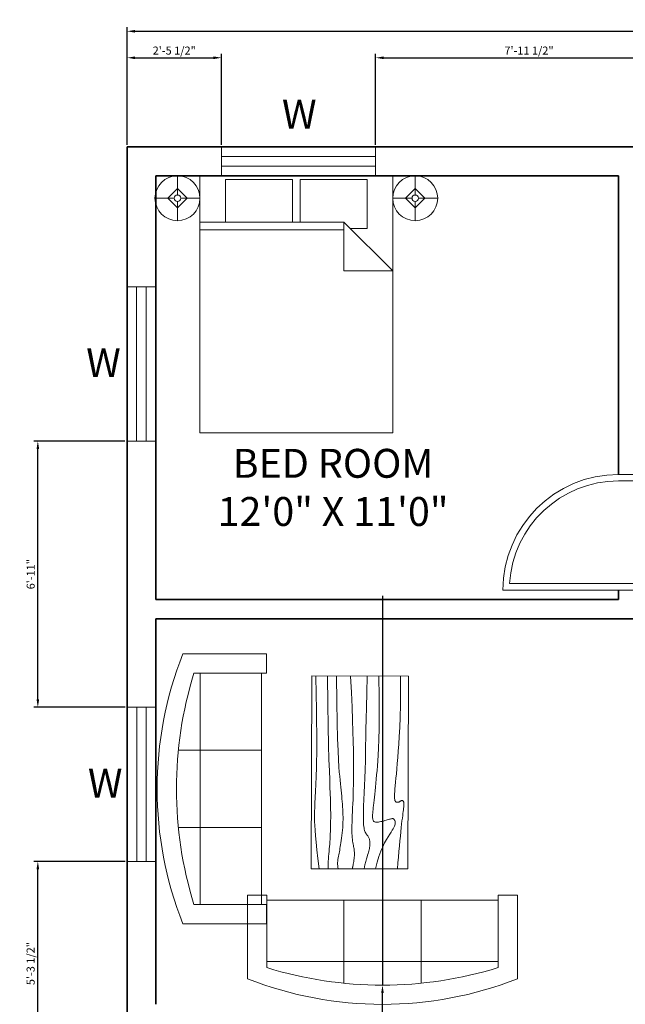
# Model space of a CAD drawing. Units: inches. Extents: x 1025 to 3479, y 1594 to 2212.
# Tile 2 of 9: x 1766 to 1954, y 1843 to 2150. Entities that reach past the tile are written whole.
import ezdxf

# ---------------------------------------------------------------- set-up
doc = ezdxf.new("R2010")
doc.units = ezdxf.units.IN
for name, color, linetype, lineweight in [('A-ANNO-DIMS', 1, 'Continuous', 18), ('A-ANNO-TEXT', 7, 'Continuous', 18), ('A-AREA-IDEN', 4, 'Continuous', 18), ('A-DOOR', 4, 'Continuous', 18), ('A-FURN', 8, 'Continuous', 13), ('A-GLAZ', 3, 'Continuous', 18), ('A-WALL', 7, 'Continuous', 35)]:
    doc.layers.add(name, color=color, linetype=linetype, lineweight=lineweight)
doc.styles.get("Standard").update_dxf_attribs({"font": 'arial.ttf'})
doc.dimstyles.new('ISO-25', dxfattribs={"dimtxt": 2.5, "dimasz": 2.5, "dimexe": 1.25, "dimexo": 0.625, "dimtad": 1, "dimdec": 0, "dimlunit": 3, "dimtxsty": 'Standard', "dimcen": 2.5, "dimadec": 0, "dimazin": 0, "dimtfac": 1, "dimtdec": 0, "dimtmove": 0, "dimatfit": 3, "dimfxl": 1, "dimarcsym": 0})

# ---------------------------------------------------------------- blocks, each defined once
blk = doc.blocks.new('*D1')
at = {"layer": 'A-ANNO-DIMS', "color": 0, "lineweight": -2, "transparency": 16777216}
for p, q in [((1799.1, 2111.11), (1799.1, 2147.74)), ((1801.6, 2146.49), (2156.6, 2146.49)), ((2159.1, 2111.11), (2159.1, 2147.74))]:
    blk.add_line(p, q, dxfattribs=at)
at = {"layer": 'A-ANNO-DIMS', "color": 0, "transparency": 16777216}
for points in [[(1801.6, 2146.9), (1801.6, 2146.07), (1799.1, 2146.49)], [(2156.6, 2146.9), (2156.6, 2146.07), (2159.1, 2146.49)]]:
    blk.add_solid(points, dxfattribs=at)
at = {"layer": 'Defpoints', "color": 0, "transparency": 16777216}
for p in [(2159.1, 2146.49), (1799.1, 2110.49), (2159.1, 2110.49)]:
    blk.add_point(p, dxfattribs=at)
at = {"layer": 'A-ANNO-DIMS', "color": 0, "transparency": 16777216, "insert": (1979.1, 2148.39), "char_height": 2.5, "attachment_point": 5}
blk.add_mtext("30'", dxfattribs=at)
blk = doc.blocks.new('Sofa - Roundback 7 ft.')
for p, q in [((-12.00002, -32.4421), (-12.00003, -6.5971)), ((11.99997, -32.4421), (11.99998, -6.5971)), ((-36.000027, -34), (-36.000027, -11.4696)), ((35.99998, -34), (35.99998, -11.4696)), ((-35.999844, -13.3819), (35.9998, -13.3819)), ((-36.000027, -32.4421), (35.99998, -32.4421))]:
    blk.add_line(p, q)
for points in [[(-36.000027, -34), (-42.000027, -34), (-42.000027, -8)], [(41.99998, -8), (41.99998, -34), (35.99998, -34)]]:
    blk.add_lwpolyline(points)
for centre, radius, start, end in [((0, -114.25), 114.25, 68.43141, 111.5686), ((-0.00001, -127.1968), 121.1968, 72.72033, 107.2797)]:
    blk.add_arc(centre, radius, start, end)
blk = doc.blocks.new('Table - Rectangular Woodgrain 60 x 30 in.')
for p, q in [((0, 0), (0, -30)), ((60, 0), (0, 0)), ((60, -30), (60, 0)), ((0, -30), (60, -30))]:
    blk.add_line(p, q)
for points in [[(0, -2.4), (4.8155, -2.418), (9.0302, -2.4688), (12.709, -2.5477), (15.9167, -2.65), (18.7181, -2.7711), (21.1781, -2.9063), (23.3616, -3.0508), (25.3333, -3.2), (27.1477, -3.3495), (28.8172, -3.4958), (30.3437, -3.636), (31.7291, -3.7667), (32.9756, -3.8849), (34.0849, -3.9875), (35.059, -4.0714), (35.9, -4.1334), (36.6114, -4.1711), (37.2041, -4.1854), (37.6906, -4.1779), (38.0833, -4.15), (38.3948, -4.1034), (38.6375, -4.0396), (38.8239, -3.9602), (38.9666, -3.8667), (39.0764, -3.7608), (39.1573, -3.6448), (39.2116, -3.521), (39.2416, -3.3917), (39.2498, -3.2593), (39.2385, -3.1261), (39.21, -2.9944), (39.1666, -2.8667), (39.111, -2.7447), (39.0468, -2.6281), (38.978, -2.5163), (38.9083, -2.4083), (38.8418, -2.3035), (38.7823, -2.201), (38.7337, -2.1001), (38.7, -2), (38.6844, -1.9003), (38.6875, -1.8021), (38.7094, -1.707), (38.75, -1.6167), (38.8094, -1.5326), (38.8875, -1.4563), (38.9844, -1.3893), (39.1, -1.3333), (39.2351, -1.2896), (39.3937, -1.2583), (39.5804, -1.2396), (39.8, -1.2333), (40.057, -1.2396), (40.3562, -1.2583), (40.7023, -1.2896), (41.1, -1.3333), (41.5547, -1.3895), (42.0755, -1.4573), (42.6721, -1.5361), (43.3542, -1.625), (44.1316, -1.7233), (45.014, -1.8302), (46.0114, -1.9449), (47.1333, -2.0667), (48.3862, -2.1947), (49.7625, -2.3281), (51.2513, -2.4663), (52.8416, -2.6083), (54.5226, -2.7535), (56.2833, -2.9011), (58.1127, -3.0501), (60, -3.2)], [(0, -9.2), (6.5759, -9.0858), (11.9385, -9.0365), (16.2527, -9.0418), (19.6833, -9.0917), (22.3952, -9.1759), (24.5531, -9.2844), (26.322, -9.4069), (27.8666, -9.5333), (29.3241, -9.6553), (30.7203, -9.7719), (32.0532, -9.8837), (33.3208, -9.9917), (34.5213, -10.0965), (35.6526, -10.199), (36.7128, -10.2999), (37.7, -10.4), (38.6129, -10.4996), (39.4531, -10.5969), (40.223, -10.6895), (40.925, -10.775), (41.5613, -10.8512), (42.1344, -10.9156), (42.6465, -10.966), (43.1, -11), (43.4976, -11.0158), (43.8437, -11.0136), (44.143, -10.9942), (44.4, -10.9583), (44.6195, -10.9069), (44.8062, -10.8406), (44.9648, -10.7603), (45.1, -10.6667), (45.2155, -10.5598), (45.3114, -10.4365), (45.3871, -10.2929), (45.4416, -10.125), (45.4743, -9.929), (45.4844, -9.7011), (45.4709, -9.4371), (45.4333, -9.1333), (45.3716, -8.7883), (45.2896, -8.4104), (45.1919, -8.0107), (45.0833, -7.6), (44.9685, -7.1893), (44.8521, -6.7896), (44.7388, -6.4117), (44.6333, -6.0667), (44.54, -5.7628), (44.4614, -5.4979), (44.4001, -5.2675), (44.3583, -5.0667), (44.3384, -4.8909), (44.3427, -4.7354), (44.3736, -4.5956), (44.4333, -4.4667), (44.5236, -4.3453), (44.6427, -4.2333), (44.7884, -4.1339), (44.9583, -4.05), (45.1501, -3.9849), (45.3614, -3.9417), (45.59, -3.9234), (45.8333, -3.9333), (46.0915, -3.9749), (46.3734, -4.0531), (46.6906, -4.1736), (47.0542, -4.3417), (47.4756, -4.5629), (47.9661, -4.8427), (48.5372, -5.1866), (49.2, -5.6), (49.9676, -6.0844), (50.8594, -6.625), (51.8965, -7.2031), (53.1, -7.8), (54.491, -8.3969), (56.0906, -8.975), (57.9199, -9.5156), (60, -10)], [(0, -12.8), (5.1847, -12.9322), (9.6213, -13.0323), (13.3963, -13.1059), (16.5958, -13.1583), (19.3063, -13.1952), (21.614, -13.2219), (23.6054, -13.2439), (25.3666, -13.2667), (26.9728, -13.2947), (28.4531, -13.3281), (29.8256, -13.3663), (31.1083, -13.4083), (32.3191, -13.4535), (33.476, -13.501), (34.597, -13.5501), (35.7, -13.6), (36.7984, -13.6497), (37.8875, -13.6979), (38.9578, -13.743), (40, -13.7833), (41.0047, -13.8174), (41.9625, -13.8438), (42.864, -13.8607), (43.7, -13.8667), (44.4631, -13.8604), (45.1552, -13.8417), (45.7801, -13.8104), (46.3416, -13.7667), (46.8439, -13.7104), (47.2906, -13.6417), (47.6858, -13.5604), (48.0333, -13.4667), (48.3375, -13.3608), (48.6042, -13.2448), (48.8396, -13.121), (49.05, -12.9917), (49.2417, -12.8593), (49.4208, -12.7261), (49.5937, -12.5944), (49.7667, -12.4667), (49.9452, -12.3451), (50.1323, -12.2313), (50.3303, -12.1268), (50.5416, -12.0333), (50.7686, -11.9524), (51.0135, -11.8854), (51.2788, -11.8341), (51.5666, -11.8), (51.8785, -11.7843), (52.2116, -11.7865), (52.562, -11.8059), (52.926, -11.8417), (53.2998, -11.8931), (53.6795, -11.9594), (54.0614, -12.0397), (54.4416, -12.1333), (54.8223, -12.2401), (55.2293, -12.3625), (55.6942, -12.5037), (56.2489, -12.6667), (56.9251, -12.8547), (57.7545, -13.0708), (58.7689, -13.3182), (60, -13.6)], [(0, -18), (5.124, -17.7273), (9.6609, -17.5057), (13.6705, -17.3303), (17.2125, -17.1958), (20.3467, -17.0973), (23.1328, -17.0297), (25.6307, -16.9878), (27.9, -16.9667), (29.9928, -16.9617), (31.9302, -16.9703), (33.7254, -16.9907), (35.3917, -17.0208), (36.9423, -17.0588), (38.3906, -17.1026), (39.7499, -17.1503), (41.0333, -17.2), (42.2519, -17.2496), (43.4073, -17.2969), (44.4986, -17.3395), (45.525, -17.375), (46.4858, -17.4012), (47.3802, -17.4156), (48.2074, -17.416), (48.9667, -17.4), (49.6583, -17.3662), (50.2872, -17.3167), (50.8595, -17.2547), (51.3812, -17.1833), (51.8584, -17.1057), (52.2971, -17.025), (52.7034, -16.9443), (53.0833, -16.8667), (53.443, -16.7951), (53.789, -16.7313), (54.128, -16.6768), (54.4666, -16.6334), (54.8115, -16.6024), (55.1693, -16.5854), (55.5465, -16.5841), (55.95, -16.6), (56.3828, -16.6337), (56.8346, -16.6823), (57.2915, -16.7418), (57.7396, -16.8084), (58.165, -16.878), (58.5539, -16.9469), (58.8924, -17.0111), (59.1666, -17.0667), (59.3679, -17.1107), (59.5078, -17.1438), (59.6032, -17.1675), (59.6708, -17.1833), (59.7275, -17.193), (59.7901, -17.1979), (59.8753, -17.1998), (60, -17.2)], [(0, -22.4), (8.0098, -22.2501), (14.4094, -22.1011), (19.4168, -21.9535), (23.25, -21.8083), (26.1269, -21.6663), (28.2656, -21.5281), (29.884, -21.3947), (31.2, -21.2667), (32.3967, -21.1448), (33.5172, -21.0292), (34.5697, -20.9198), (35.5625, -20.8167), (36.5037, -20.7198), (37.4015, -20.6292), (38.2642, -20.5448), (39.1, -20.4667), (39.9164, -20.3951), (40.7187, -20.3313), (41.5117, -20.2768), (42.3, -20.2333), (43.0883, -20.2024), (43.8812, -20.1854), (44.6836, -20.1841), (45.5, -20.2), (46.3328, -20.234), (47.1747, -20.2844), (48.0163, -20.3488), (48.8479, -20.425), (49.66, -20.5106), (50.4429, -20.6031), (51.1872, -20.7004), (51.8833, -20.8), (52.5246, -20.8999), (53.1166, -20.9995), (53.6681, -21.0983), (54.1875, -21.1958), (54.6834, -21.2919), (55.1646, -21.3859), (55.6394, -21.4777), (56.1167, -21.5667), (56.6028, -21.6515), (57.0961, -21.7266), (57.5929, -21.7852), (58.0896, -21.8208), (58.5823, -21.8268), (59.0674, -21.7964), (59.5412, -21.723), (60, -21.6)], [(0, -25.2), (8.6355, -25.0504), (15.7026, -24.9031), (21.4049, -24.7606), (25.9458, -24.625), (29.529, -24.4988), (32.3578, -24.3844), (34.6359, -24.284), (36.5667, -24.2), (38.3213, -24.1341), (39.9417, -24.0854), (41.437, -24.0523), (42.8167, -24.0333), (44.0901, -24.0268), (45.2667, -24.0313), (46.3557, -24.0451), (47.3667, -24.0667), (48.309, -24.0947), (49.1928, -24.1287), (50.0284, -24.168), (50.826, -24.2125), (51.5959, -24.2617), (52.3483, -24.3151), (53.0935, -24.3725), (53.8417, -24.4334), (54.6009, -24.497), (55.3699, -24.561), (56.1454, -24.6226), (56.9239, -24.6792), (57.7021, -24.7279), (58.4764, -24.7662), (59.2435, -24.7911), (60, -24.8)], [(0, -28.8), (5.6867, -28.6681), (10.45, -28.5698), (14.407, -28.5012), (17.675, -28.4584), (20.3711, -28.4374), (22.6125, -28.4344), (24.5164, -28.4455), (26.2, -28.4667), (27.762, -28.4947), (29.2276, -28.5281), (30.6033, -28.5663), (31.8958, -28.6084), (33.1118, -28.6535), (34.2578, -28.7011), (35.3405, -28.7501), (36.3666, -28.8), (37.3443, -28.8497), (38.288, -28.8974), (39.2137, -28.9412), (40.1375, -28.9792), (41.0753, -29.0093), (42.0432, -29.0297), (43.0572, -29.0384), (44.1333, -29.0333), (45.2936, -29.0114), (46.5843, -28.9641), (48.0579, -28.8816), (49.7666, -28.7542), (51.7629, -28.5721), (54.0989, -28.3255), (56.8272, -28.0048), (60, -27.6)]]:
    blk.add_lwpolyline(points)
blk = doc.blocks.new('Bed - Queen')
for p, q in [((0, -80.00003), (0, 0)), ((0, 0), (59.99999, 0)), ((59.99999, 0), (59.99999, -80.00003)), ((7.99999, -1.2), (28.79998, -1.2)), ((7.99999, -14.4), (7.99999, -1.2)), ((28.79998, -1.2), (28.79998, -14.4)), ((31.19999, -1.2), (51.99999, -1.2)), ((31.19999, -14.4), (31.19999, -1.2)), ((51.99999, -1.2), (51.99999, -16.4)), ((0, -14.4), (44.8, -14.4)), ((59.99999, -29.6), (44.8, -14.4)), ((44.8, -14.4), (44.8, -29.6)), ((44.8, -16.8), (0, -16.8)), ((51.99999, -16.4), (46.79936, -16.4)), ((44.8, -29.6), (59.99999, -29.6)), ((59.99999, -80.00003), (0, -80.00003))]:
    blk.add_line(p, q)
blk = doc.blocks.new('Lamp - Table')
for p, q in [((0, 7), (0, 1)), ((-1, 0), (-7, 0)), ((0, 3), (-3, 0)), ((-3, 0), (0, -3)), ((3, 0), (0, 3)), ((0, -3), (3, 0)), ((1, 0), (7, 0)), ((0, -1), (0, -7))]:
    blk.add_line(p, q)
for radius in [7, 1]:
    blk.add_circle((0, 0), radius)
blk = doc.blocks.new('WIN-48IN')
for p, q in [((0, 48), (0, 0)), ((9, 48), (0, 48)), ((3, 48), (3, 0)), ((6, 0), (6, 48)), ((9, 0), (9, 48)), ((0, 0), (9, 0))]:
    blk.add_line(p, q)
blk = doc.blocks.new('DOOR-SWING-36IN')
for p, q in [((0, 36), (6, 36)), ((0, 34), (6, 34)), ((0, 2), (6, 2)), ((6, 0), (0, 0)), ((6, 2), (39.94, 2)), ((6, 0), (42, 0))]:
    blk.add_line(p, q)
for radius, start in [(36, 0), (34, 3.3723)]:
    blk.add_arc((6, 0), radius, start, 90)
blk = doc.blocks.new('*D49')
at = {"layer": 'A-ANNO-DIMS', "color": 0, "lineweight": -2, "transparency": 16777216}
for p, q in [((1799.1, 2111.11), (1799.1, 2139.49)), ((1801.6, 2138.24), (1825.98, 2138.24)), ((1828.48, 2111.11), (1828.48, 2139.49))]:
    blk.add_line(p, q, dxfattribs=at)
at = {"layer": 'A-ANNO-DIMS', "color": 0, "transparency": 16777216}
for points in [[(1801.6, 2138.65), (1801.6, 2137.82), (1799.1, 2138.24)], [(1825.98, 2138.65), (1825.98, 2137.82), (1828.48, 2138.24)]]:
    blk.add_solid(points, dxfattribs=at)
at = {"layer": 'Defpoints', "color": 0, "transparency": 16777216}
for p in [(1828.48, 2138.24), (1799.1, 2110.49), (1828.48, 2110.49)]:
    blk.add_point(p, dxfattribs=at)
at = {"layer": 'A-ANNO-DIMS', "color": 0, "transparency": 16777216, "insert": (1813.79, 2140.15), "char_height": 2.5, "attachment_point": 5}
blk.add_mtext('2\'-5 1/2"', dxfattribs=at)
blk = doc.blocks.new('*D50')
at = {"layer": 'A-ANNO-DIMS', "color": 0, "lineweight": -2, "transparency": 16777216}
for p, q in [((1876.48, 2111.11), (1876.48, 2139.49)), ((1878.98, 2138.24), (1969.43, 2138.24)), ((1971.93, 2111.11), (1971.93, 2139.49))]:
    blk.add_line(p, q, dxfattribs=at)
at = {"layer": 'A-ANNO-DIMS', "color": 0, "transparency": 16777216}
for points in [[(1878.98, 2138.65), (1878.98, 2137.82), (1876.48, 2138.24)], [(1969.43, 2138.65), (1969.43, 2137.82), (1971.93, 2138.24)]]:
    blk.add_solid(points, dxfattribs=at)
at = {"layer": 'Defpoints', "color": 0, "transparency": 16777216}
for p in [(1971.93, 2138.24), (1876.48, 2110.49), (1971.93, 2110.49)]:
    blk.add_point(p, dxfattribs=at)
at = {"layer": 'A-ANNO-DIMS', "color": 0, "transparency": 16777216, "insert": (1924.21, 2140.15), "char_height": 2.5, "attachment_point": 5}
blk.add_mtext('7\'-11 1/2"', dxfattribs=at)
blk = doc.blocks.new('*D54')
at = {"layer": 'A-ANNO-DIMS', "color": 0, "lineweight": -2, "transparency": 16777216}
for p, q in [((1798.47, 1887.99), (1770.08, 1887.99)), ((1771.33, 1826.84), (1771.33, 1885.49)), ((1798.47, 1824.34), (1770.08, 1824.34))]:
    blk.add_line(p, q, dxfattribs=at)
at = {"layer": 'A-ANNO-DIMS', "color": 0, "transparency": 16777216}
for points in [[(1770.92, 1885.49), (1771.75, 1885.49), (1771.33, 1887.99)], [(1770.92, 1826.84), (1771.75, 1826.84), (1771.33, 1824.34)]]:
    blk.add_solid(points, dxfattribs=at)
at = {"layer": 'Defpoints', "color": 0, "transparency": 16777216}
for p in [(1771.33, 1887.99), (1799.1, 1887.99), (1799.1, 1824.34)]:
    blk.add_point(p, dxfattribs=at)
at = {"layer": 'A-ANNO-DIMS', "color": 0, "transparency": 16777216, "insert": (1769.41, 1856.16), "char_height": 2.5, "attachment_point": 5, "rotation": 90}
blk.add_mtext('5\'-3 1/2"', dxfattribs=at)
blk = doc.blocks.new('*D55')
at = {"layer": 'A-ANNO-DIMS', "color": 0, "lineweight": -2, "transparency": 16777216}
for p, q in [((1798.46, 2018.87), (1770.08, 2018.87)), ((1771.33, 1938.49), (1771.33, 2016.37)), ((1798.47, 1935.99), (1770.08, 1935.99))]:
    blk.add_line(p, q, dxfattribs=at)
at = {"layer": 'A-ANNO-DIMS', "color": 0, "transparency": 16777216}
for points in [[(1770.92, 2016.37), (1771.75, 2016.37), (1771.33, 2018.87)], [(1770.92, 1938.49), (1771.75, 1938.49), (1771.33, 1935.99)]]:
    blk.add_solid(points, dxfattribs=at)
at = {"layer": 'Defpoints', "color": 0, "transparency": 16777216}
for p in [(1771.33, 2018.87), (1799.08, 2018.87), (1799.1, 1935.99)]:
    blk.add_point(p, dxfattribs=at)
at = {"layer": 'A-ANNO-DIMS', "color": 0, "transparency": 16777216, "insert": (1769.43, 1977.43), "char_height": 2.5, "attachment_point": 5, "rotation": 90}
blk.add_mtext('6\'-11"', dxfattribs=at)
blk = doc.blocks.new('*D90')
at = {"layer": 'A-ANNO-DIMS', "color": 0, "lineweight": -2, "transparency": 16777216}
for p, q in [((1878.6, 1970.65), (1878.6, 1849.46)), ((1878.6, 1767.94), (1878.6, 1846.96))]:
    blk.add_line(p, q, dxfattribs=at)
at = {"layer": 'A-ANNO-DIMS', "color": 0, "transparency": 16777216}
blk.add_solid([(1879.02, 1846.96), (1878.18, 1846.96), (1878.6, 1849.46)], dxfattribs=at)
at = {"layer": 'Defpoints', "color": 0, "transparency": 16777216}
for p in [(1878.6, 1970.65), (1878.6, 1849.46)]:
    blk.add_point(p, dxfattribs=at)
at = {"layer": 'A-ANNO-DIMS', "color": 0, "transparency": 16777216, "insert": (1880.5, 1776.74), "char_height": 2.5, "attachment_point": 5, "rotation": 270.0002}
blk.add_mtext('5X R10\'-1"', dxfattribs=at)

msp = doc.modelspace()

# ---------------------------------------------------------------- linework, layer by layer
at = {"layer": 'A-DOOR'}
msp.add_line((1958.1, 1972.49), (1952.1, 1972.49), dxfattribs=at)
at = {"layer": 'A-WALL'}
for p, q in [((1799.1, 2110.49), (2159.1, 2110.49)), ((1799.1, 1670.49), (1799.1, 2110.49)), ((1799.1, 1670.49), (1799.1, 2110.49)), ((1808.1, 2101.49), (1952.1, 2101.49)), ((1808.1, 1969.49), (1808.1, 2101.49)), ((1952.1, 2008.49), (1952.1, 2101.49)), ((1952.1, 2008.49), (1952.1, 2101.49)), ((1952.1, 2008.49), (1952.1, 2101.49)), ((1952.1, 1969.49), (1952.1, 1972.49)), ((1952.1, 1969.49), (1952.1, 1972.49)), ((1952.1, 1969.49), (1952.1, 1972.49)), ((1808.1, 1969.49), (1952.1, 1969.49)), ((1808.1, 1963.49), (1958.1, 1963.49)), ((1808.1, 1843.49), (1808.1, 1963.49))]:
    msp.add_line(p, q, dxfattribs=at)

# ---------------------------------------------------------------- block references
at = {"layer": 'A-DOOR', "extrusion": (0, 0, -1), "zscale": -1}
msp.add_blockref('DOOR-SWING-36IN', (-1958.1, 1972.49), dxfattribs=at)
at = {"layer": 'A-FURN'}
for name, p in [('Lamp - Table', (1814.79, 2094.49)), ('Bed - Queen', (1821.79, 2101.49)), ('Lamp - Table', (1888.79, 2094.49))]:
    msp.add_blockref(name, p, dxfattribs=at)
for name, p, rotation in [('Sofa - Roundback 7 ft.', (1808.46, 1910.58), 90), ('Table - Rectangular Woodgrain 60 x 30 in.', (1886.66, 1945.62), 269.8036337053011), ('Sofa - Roundback 7 ft.', (1878.6, 1843.46), 180)]:
    msp.add_blockref(name, p, dxfattribs=dict(at, rotation=rotation))
at = {"layer": 'A-GLAZ', "rotation": 269.9999999999988}
msp.add_blockref('WIN-48IN', (1828.48, 2110.49), dxfattribs=at)
at = {"layer": 'A-GLAZ'}
for p in [(1799.08, 2018.87), (1799.1, 1887.99)]:
    msp.add_blockref('WIN-48IN', p, dxfattribs=at)

# ---------------------------------------------------------------- texts
at = {"layer": 'A-ANNO-TEXT', "char_height": 9, "attachment_point": 1}
for insert in [(1844.77, 2125.14), (1783.82, 2047.8), (1784.36, 1916.88)]:
    msp.add_mtext_dynamic_manual_height_columns('\\pxqc;W', width=15.8719, gutter_width=12.5, heights=[0], dxfattribs=dict(at, insert=insert))
at = {"layer": 'A-AREA-IDEN', "insert": (1816.6, 2016.45), "char_height": 9, "attachment_point": 1}
msp.add_mtext_dynamic_manual_height_columns('\\pxqc;BED ROOM \\P12\'0" X 11\'0"', width=93.2353, gutter_width=12.5, heights=[0], dxfattribs=at)

# ---------------------------------------------------------------- dimensions: what is measured, and where the dimension line sits
at = {"layer": 'A-ANNO-DIMS'}
for base, p1, p2, override, picture, middle in [((2159.1, 2146.49), (1799.1, 2110.49), (2159.1, 2110.49), {"dimclrd": 0, "dimclre": 0, "dimclrt": 0}, '*D1', (1979.1, 2148.39)), ((1828.48, 2138.24), (1799.1, 2110.49), (1828.48, 2110.49), {"dimdec": 1, "dimlfac": 1, "dimrnd": 0, "dimzin": 1, "dimdsep": 46, "dimlunit": 4, "dimfrac": 2}, '*D49', (1813.79, 2140.15)), ((1971.9348, 2138.2355), (1876.4813, 2110.4855), (1971.9348, 2110.4855), {"dimdec": 1, "dimlfac": 1, "dimrnd": 0, "dimzin": 1, "dimdsep": 46, "dimlunit": 4, "dimfrac": 2}, '*D50', (1924.208, 2140.1532))]:
    dim = msp.add_linear_dim(base=base, p1=p1, p2=p2, dimstyle='ISO-25', override=override, dxfattribs=at)
    dim.commit()
    dim.dimension.update_dxf_attribs({"geometry": picture, "text_midpoint": middle})
for base, p1, p2, picture, middle in [((1771.33, 2018.87), (1799.1, 1935.99), (1799.08, 2018.87), '*D55', (1769.43, 1977.43)), ((1771.332537, 1887.985569), (1799.099068, 1824.335569), (1799.099068, 1887.985569), '*D54', (1769.41405132, 1856.160569))]:
    dim = msp.add_linear_dim(base=base, p1=p1, p2=p2, angle=90, dimstyle='ISO-25', override={"dimdec": 1, "dimlfac": 1, "dimrnd": 0, "dimzin": 1, "dimdsep": 46, "dimlunit": 4, "dimfrac": 2}, dxfattribs=at)
    dim.commit()
    dim.dimension.update_dxf_attribs({"geometry": picture, "text_midpoint": middle})
dim = msp.add_radius_dim(center=(1878.6, 1970.65), mpoint=(1878.6, 1849.46), text='5X <>', dimstyle='ISO-25', override={"dimdec": 1, "dimlfac": 1, "dimrnd": 0, "dimzin": 1, "dimdsep": 46, "dimlunit": 4, "dimfrac": 2}, dxfattribs=at)
dim.commit()
dim.dimension.update_dxf_attribs({"geometry": '*D90', "text_midpoint": (1878.6, 1776.74), "dimtype": 164})

doc.saveas('drawing.dxf')
